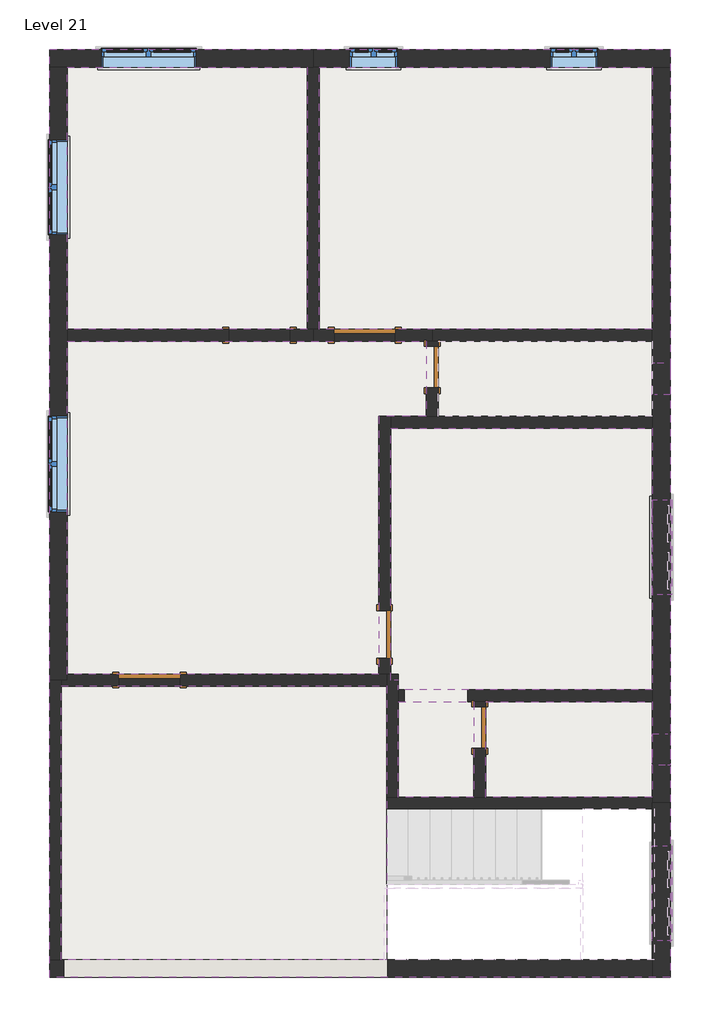
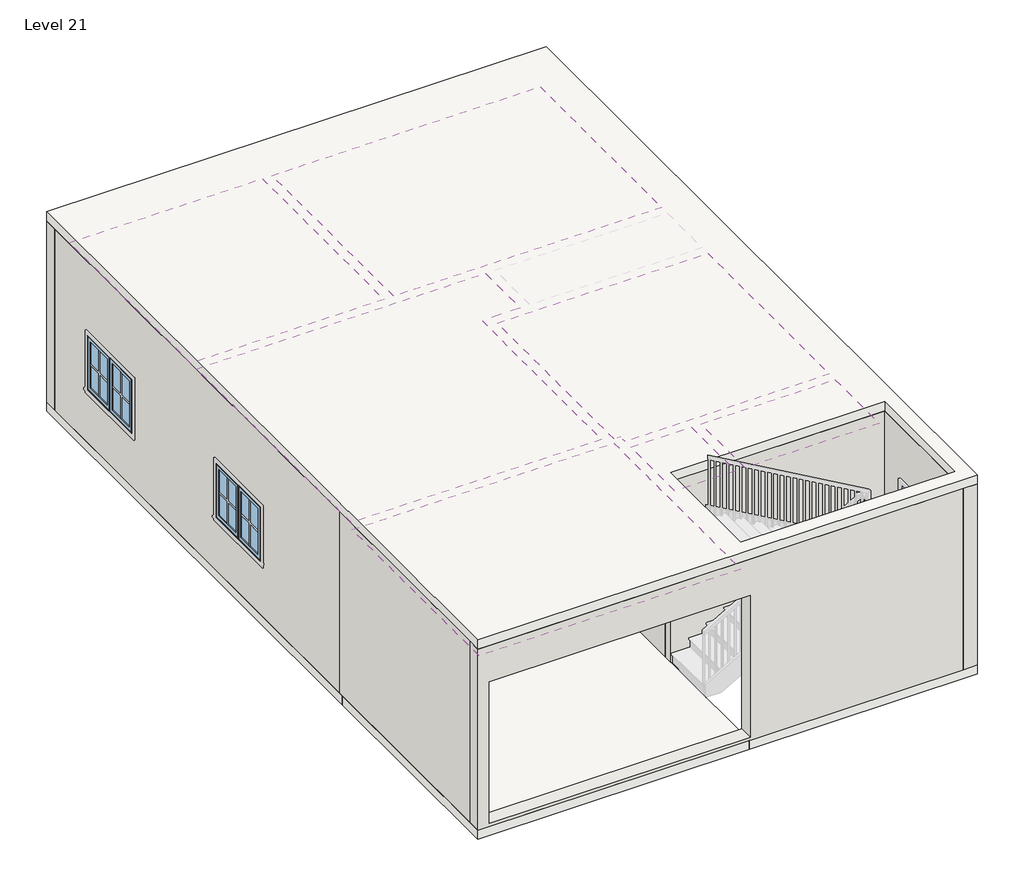
# One storey, part 1 of 2: 27 walls, 13 windows, 7 coverings, 6 doors, 3 slabs.
# Revit data of these elements (continued)
# Element 47 (IfcWindow, "Window-Casement-Double : 3'") (continued)
#   Materials on its faces: "Wood - Stained", "Glass", "Clad - White"
# Element 48 (IfcWindow, "Window-Casement-Double : 3'")
#   Mark = "90"
#   Window Inset = 0' - 0"
#   Interior Wall Closure = 0' - 2 1/4"
#   Frame Extension = 0' - 0 1/4"
#   Exterior Wall Closure = 0' - 1 1/4"
#   Interior Trim Visibility = yes
#   Exterior Trim Visibility = yes
#   Phase Created = New Construction
#   Materials on its faces: "Wood - Stained", "Glass", "Clad - White"
# Element 49 (IfcWindow, "Window-Casement-Double : 3'")
#   Mark = "91"
#   Window Inset = 0' - 0"
#   Interior Wall Closure = 0' - 2 1/4"
#   Frame Extension = 0' - 0 1/4"
#   Exterior Wall Closure = 0' - 1 1/4"
#   Interior Trim Visibility = yes
#   Exterior Trim Visibility = yes
#   Phase Created = New Construction
#   Materials on its faces: "Wood - Stained", "Glass", "Clad - White"
# Element 50 (IfcWindow, "Window-Casement-Double : 4'")
#   Mark = "79"
#   Window Inset = 0' - 0"
#   Interior Wall Closure = 0' - 2 1/4"
#   Frame Extension = 0' - 0 1/4"
#   Exterior Wall Closure = 0' - 1 1/4"
#   Interior Trim Visibility = yes
#   Exterior Trim Visibility = yes
#   Phase Created = New Construction
#   Materials on its faces: "Wood - Stained", "Glass", "Clad - White"
# Element 51 (IfcWindow, "Window-Casement-Double : 4'")
#   Mark = "80"
#   Window Inset = 0' - 0"
#   Interior Wall Closure = 0' - 2 1/4"
#   Frame Extension = 0' - 0 1/4"
#   Exterior Wall Closure = 0' - 1 1/4"
#   Interior Trim Visibility = yes
#   Exterior Trim Visibility = yes
#   Phase Created = New Construction
#   Materials on its faces: "Wood - Stained", "Glass", "Clad - White"
# Element 52 (IfcWindow, "Window-Casement-Double : 4'")
#   Mark = "81"
#   Window Inset = 0' - 0"
#   Interior Wall Closure = 0' - 2 1/4"
#   Frame Extension = 0' - 0 1/4"
#   Exterior Wall Closure = 0' - 1 1/4"
#   Interior Trim Visibility = yes
#   Exterior Trim Visibility = yes
#   Phase Created = New Construction
#   Materials on its faces: "Wood - Stained", "Glass", "Clad - White"
# Element 53 (IfcWindow, "Window-Casement-Double : 4'")
#   Mark = "82"
#   Window Inset = 0' - 0"
#   Interior Wall Closure = 0' - 2 1/4"
#   Frame Extension = 0' - 0 1/4"
#   Exterior Wall Closure = 0' - 1 1/4"
#   Interior Trim Visibility = yes
#   Exterior Trim Visibility = yes
#   Phase Created = New Construction
#   Materials on its faces: "Wood - Stained", "Glass", "Clad - White"
# Element 54 (IfcWindow, "Window-Casement-Double : 4'")
#   Mark = "83"
#   Window Inset = 0' - 0"
#   Interior Wall Closure = 0' - 2 1/4"
#   Frame Extension = 0' - 0 1/4"
#   Exterior Wall Closure = 0' - 1 1/4"
#   Interior Trim Visibility = yes
#   Exterior Trim Visibility = yes
#   Phase Created = New Construction
#   Materials on its faces: "Wood - Stained", "Glass", "Clad - White"
# Element 55 (IfcWindow, "Window-Casement-Double : 4'")
#   Mark = "88"
#   Window Inset = 0' - 0"
#   Interior Wall Closure = 0' - 2 1/4"
#   Frame Extension = 0' - 0 1/4"
#   Exterior Wall Closure = 0' - 1 1/4"
#   Interior Trim Visibility = yes
#   Exterior Trim Visibility = yes
#   Phase Created = New Construction
#   Materials on its faces: "Wood - Stained", "Glass", "Clad - White"
# Element 56 (IfcWindow, "Window-Casement-Double : 4'")
#   Mark = "89"
#   Window Inset = 0' - 0"
#   Interior Wall Closure = 0' - 2 1/4"
#   Frame Extension = 0' - 0 1/4"
#   Exterior Wall Closure = 0' - 1 1/4"
#   Interior Trim Visibility = yes
#   Exterior Trim Visibility = yes
#   Phase Created = New Construction
#   Materials on its faces: "Wood - Stained", "Glass", "Clad - White"
# Materials
#   "Default": colour RGB 127 127 127, transparency 0, Cost = 0
#   "Acoustic Ceiling Tile 24 x 48": class "Generic", colour RGB 229 229 229, transparency 0, Description = "Acoustic Ceiling Tile 24 x 48", Cost = 0
#   "Door - Panel": class "Wood", colour RGB 210 159 95, transparency 0, Cost = 0
#   "Door - Frame": colour RGB 118 70 51, transparency 0, Cost = 0
#   "Glass": class "Glass", colour RGB 0 128 192, transparency 0.75, Description = "Soda Lime Glass", Cost = 0
#   "Sash": class "Wood", colour RGB 224 178 126, transparency 0, Cost = 0
#   "Wood - Stained": class "Wood", colour RGB 224 178 126, transparency 0, Cost = 0
#   "Clad - White": class "Wood", colour RGB 242 242 238, transparency 0, Cost = 0
#   "Default Floor": colour RGB 128 128 128, transparency 0, Cost = 0
#   "TILE": class "Generic", colour RGB 120 120 120, transparency 0, Cost = 0
#   "Grass": class "Generic", colour RGB 104 137 66, transparency 0, Description = "Physical material.", Cost = 0
#   "Default Wall": colour RGB 128 128 128, transparency 0, Cost = 0
#   "WALL PAINT 4": class "Generic", colour RGB 120 120 120, transparency 0, Cost = 0
#   "MARBLE": class "Generic", colour RGB 120 120 120, transparency 0, Cost = 0
#   "WALL PAINT 5": class "Generic", colour RGB 120 120 120, transparency 0, Cost = 0
#   "WALL PAINT 2": class "Generic", colour RGB 120 120 120, transparency 0, Cost = 0
#   "WALL PAINT 3": class "Generic", colour RGB 120 120 120, transparency 0, Cost = 0
#   "WALL PAINT 1": class "Generic", colour RGB 120 120 120, transparency 0, Cost = 0
